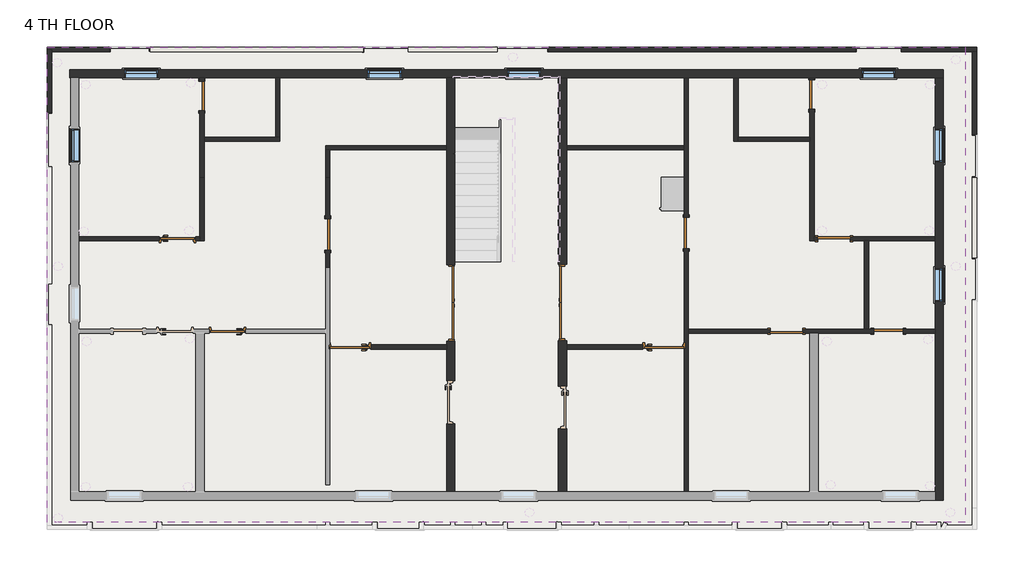
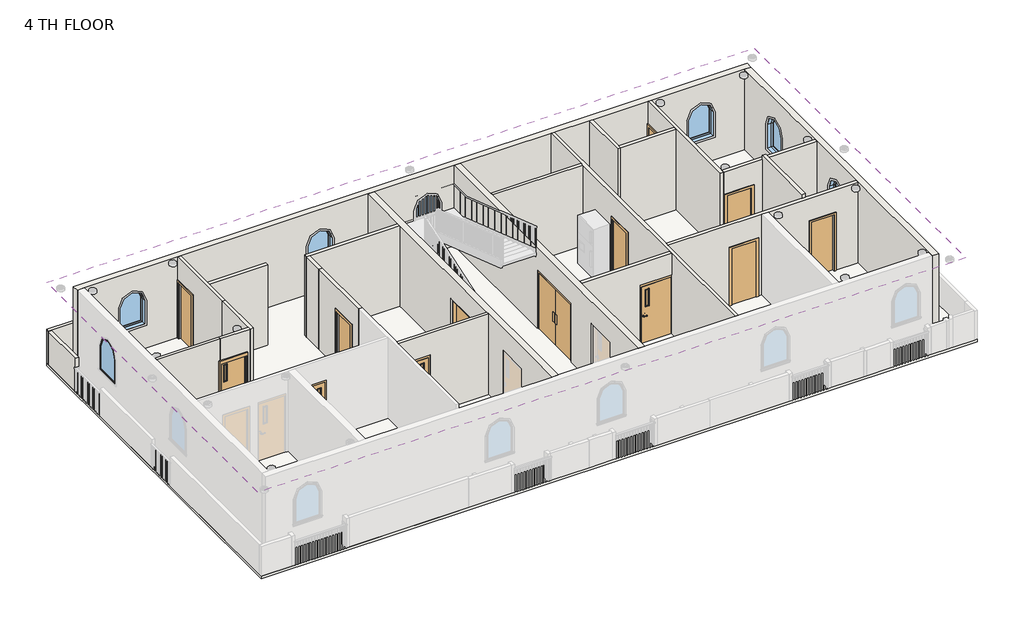
# One storey, part 2 of 7: 32 walls, 13 doors, 7 windows, 1 covering, 1 slab.
"""IFC4 building model written with IfcOpenShell, lengths in millimetres."""

from ifc_helpers import new_model, si_unit, frame, origin, place, context, project, spatial, polyline, circle_curve, outline, extrude, faceted_brep, transform, mapped, element, save
from ifc_brep_helpers import plane_surface, revolved_surface, advanced_brep
from components import door_2c854dd0, door_cf1f2706, door_4f5842df, door_passage_single_vision_lite_3_x7_440dd290, door_70e57c00, door_700d3439, door_8cb1b8a7, door_38851409, door_d141acb4, window_fixed_round_top_3_x_4_dee2be1c

model = new_model("IFC4")

# Units and contexts
model_context = context("Model", 3, world=origin())
ifc_project = project(units=[si_unit("LENGTHUNIT", "METRE", prefix="MILLI")], contexts=[model_context])

# Site, building, storey
site = spatial("IfcSite", under=ifc_project)
building = spatial("IfcBuilding", under=site)
storey = spatial("IfcBuildingStorey", under=building, Name="4 TH FLOOR", Elevation=12801.6)

# Covering
placement = place(None, origin())
element("IfcCovering", 1, ObjectType="2' x 4' ACT System", at=placement, inside=storey, context=model_context, shape_type="SweptSolid", body=[
    extrude(outline(polyline([(12235.5012075, 8470.0067329), (12235.5012075, -4623.6932193), (-13088.8067989, -4623.6932193), (-13088.8067989, 8470.0067329), (12235.5012075, 8470.0067329)])), frame((0.0, 0.0, 15849.6), z_axis=(0.0, 0.0, 1.0), x_axis=(1.0, 0.0, 0.0)), (0.0, 0.0, 1.0), 57.15),
])

# Doors
door_shape = door_2c854dd0(model_context)
element("IfcDoor", 2, ObjectType="Door-Passage-Double-Flush-Dbl_Acting : 6'79\" X 84\"", at=placement, inside=storey, context=model_context, shape_type="MappedRepresentation", body=[
    mapped(door_shape, transform((-1969.4487998, 1424.4578621, 12801.6), x_axis=(0.0, -1.0, 0.0), y_axis=(1.0, 0.0, 0.0), z_axis=(0.0, 0.0, 1.0))),
])
element("IfcDoor", 3, ObjectType="Door-Passage-Double-Flush-Dbl_Acting : 6'79\" X 84\"", at=placement, inside=storey, context=model_context, shape_type="MappedRepresentation", body=[
    mapped(door_shape, transform((1128.8432011, 1434.2067807, 12801.6), x_axis=(0.0, 1.0, 0.0), y_axis=(-1.0, 0.0, 0.0), z_axis=(0.0, 0.0, 1.0))),
])
door_2_shape = door_cf1f2706(model_context)
element("IfcDoor", 4, ObjectType="Door-Passage-Single-Vision_Lite : 3'6\"X7' 2", at=placement, inside=storey, context=model_context, shape_type="MappedRepresentation", body=[
    mapped(door_2_shape, transform((-4750.7487995, 211.6078621, 12801.6), x_axis=(-1.0, 0.0, 0.0), y_axis=(0.0, -1.0, 0.0), z_axis=(0.0, 0.0, 1.0))),
])
door_3_shape = door_4f5842df(model_context)
element("IfcDoor", 5, ObjectType="Door-Passage-Single-Vision_Lite : 3'6\"X7' 2", at=placement, inside=storey, context=model_context, shape_type="MappedRepresentation", body=[
    mapped(door_3_shape, transform((3923.3512082, 211.6078621, 12801.6), x_axis=(1.0, 0.0, 0.0), y_axis=(0.0, 1.0, 0.0), z_axis=(0.0, 0.0, 1.0))),
])
door_passage_single_vision_lite_3_x7_shape = door_passage_single_vision_lite_3_x7_440dd290(model_context)
element("IfcDoor", 6, ObjectType="Door-Passage-Single-Vision_Lite : 3'X7'", at=placement, inside=storey, context=model_context, shape_type="MappedRepresentation", body=[
    mapped(door_passage_single_vision_lite_3_x7_shape, transform((-9501.8462614, 3186.8067332, 12801.6), x_axis=(1.0, 0.0, 0.0), y_axis=(0.0, 1.0, 0.0), z_axis=(0.0, 0.0, 1.0))),
])
element("IfcDoor", 7, ObjectType="Door-Passage-Single-Vision_Lite : 3'X7'", at=placement, inside=storey, context=model_context, shape_type="MappedRepresentation", body=[
    mapped(door_passage_single_vision_lite_3_x7_shape, transform((-8122.5987992, 646.8067334, 12801.6), x_axis=(-1.0, 0.0, 0.0), y_axis=(0.0, -1.0, 0.0), z_axis=(0.0, 0.0, 1.0))),
])
door_4_shape = door_70e57c00(model_context)
element("IfcDoor", 8, ObjectType="Single-Flush : 2'10\" x 7'", at=placement, inside=storey, context=model_context, shape_type="MappedRepresentation", body=[
    mapped(door_4_shape, transform((-5360.3487995, 3313.8067802, 12801.6), x_axis=(0.0, -1.0, 0.0), y_axis=(1.0, 0.0, 0.0), z_axis=(0.0, 0.0, 1.0))),
])
door_5_shape = door_700d3439(model_context)
element("IfcDoor", 9, ObjectType="Single-Flush : 2'10\" x 7'", at=placement, inside=storey, context=model_context, shape_type="MappedRepresentation", body=[
    mapped(door_5_shape, transform((4532.9512082, 3351.906733, 12801.6), x_axis=(0.0, -1.0, 0.0), y_axis=(1.0, 0.0, 0.0), z_axis=(0.0, 0.0, 1.0))),
])
door_6_shape = door_8cb1b8a7(model_context)
element("IfcDoor", 10, ObjectType="Single-Flush : 2'11\"x 7'", at=placement, inside=storey, context=model_context, shape_type="MappedRepresentation", body=[
    mapped(door_6_shape, transform((8609.6512079, 3193.1567332, 12801.6), x_axis=(-1.0, 0.0, 0.0), y_axis=(0.0, -1.0, 0.0), z_axis=(0.0, 0.0, 1.0))),
])
element("IfcDoor", 11, ObjectType="Single-Flush : 2'11\"x 7'", at=placement, inside=storey, context=model_context, shape_type="MappedRepresentation", body=[
    mapped(door_6_shape, transform((7295.2012079, 640.4567334, 12801.6), x_axis=(1.0, 0.0, 0.0), y_axis=(0.0, 1.0, 0.0), z_axis=(0.0, 0.0, 1.0))),
])
door_7_shape = door_38851409(model_context)
element("IfcDoor", 12, ObjectType="Single-Flush : 2'8\"x 7'", at=placement, inside=storey, context=model_context, shape_type="MappedRepresentation", body=[
    mapped(door_7_shape, transform((-8827.4487992, 7136.5067329, 12801.6), x_axis=(0.0, 1.0, 0.0), y_axis=(-1.0, 0.0, 0.0), z_axis=(0.0, 0.0, 1.0))),
])
element("IfcDoor", 13, ObjectType="Single-Flush : 2'8\"x 7'", at=placement, inside=storey, context=model_context, shape_type="MappedRepresentation", body=[
    mapped(door_7_shape, transform((10111.5098918, 640.4567334, 12801.6), x_axis=(-1.0, 0.0, 0.0), y_axis=(0.0, -1.0, 0.0), z_axis=(0.0, 0.0, 1.0))),
])
door_8_shape = door_d141acb4(model_context)
element("IfcDoor", 14, ObjectType="Single-Flush : 2'8\"x 7'", at=placement, inside=storey, context=model_context, shape_type="MappedRepresentation", body=[
    mapped(door_8_shape, transform((8000.0512079, 7167.840939, 12801.6), x_axis=(0.0, 1.0, 0.0), y_axis=(-1.0, 0.0, 0.0), z_axis=(0.0, 0.0, 1.0))),
])

# Slab
element("IfcSlab", 15, ObjectType="LW Concrete on Metal Deck", at=placement, inside=storey, context=model_context, shape_type="SweptSolid", body=[
    extrude(outline(polyline([(12540.3012043, 8470.0067329), (12540.3012043, -4826.8932661), (-13088.8067989, -4826.8932661), (-13088.8067989, 8470.0067329), (12540.3012043, 8470.0067329)])), frame((0.0, 0.0, 12696.825), z_axis=(0.0, 0.0, 1.0), x_axis=(1.0, 0.0, 0.0)), (0.0, 0.0, 1.0), 104.775),
])

# Walls
element("IfcWall", 16, ObjectType="Generic - 4.5\"", at=placement, inside=storey, context=model_context, shape_type="SweptSolid", body=[
    extrude(outline(polyline([(15849.6, -9959.0462614), (15849.6, -12224.6987925), (12801.6, -12224.6987925), (12801.6, -10009.8462614), (15036.8, -10009.8462614), (15036.8, -9959.0462614), (15849.6, -9959.0462614)])), frame((0.0, 3136.0067332, 0.0), z_axis=(0.0, 1.0, 0.0), x_axis=(0.0, 0.0, 1.0)), (0.0, 0.0, 1.0), 114.3),
])
element("IfcWall", 17, ObjectType="Generic - 4.5\"", at=placement, inside=storey, context=model_context, shape_type="Brep", body=[
    faceted_brep([(-8884.5987992, 4875.906733, 12801.6), (-8884.5987992, 3250.3067332, 12801.6), (-8884.5987992, 3136.0067332, 12801.6), (-8884.5987992, 3136.0067332, 15849.6), (-8884.5987992, 3250.3067332, 15849.6), (-8884.5987992, 4875.906733, 15849.6), (-8770.2987992, 4875.906733, 12801.6), (-8770.2987992, 4875.906733, 15849.6), (-8770.2987992, 3136.0067332, 15849.6), (-8770.2987992, 3136.0067332, 12801.6)], [[[0, 1, 2, 3, 4, 5]], [[6, 7, 8, 9]], [[2, 1, 0, 6, 9]], [[5, 4, 3, 8, 7]], [[0, 5, 7, 6]], [[3, 2, 9, 8]]]),
])
element("IfcWall", 18, ObjectType="Generic - 4.5\"", at=placement, inside=storey, context=model_context, shape_type="SweptSolid", body=[
    extrude(outline(polyline([(15849.6, -2077.3987998), (15849.6, -5303.1987995), (15036.8, -5303.1987995), (15036.8, -4166.5487995), (12801.6, -4166.5487995), (12801.6, -2077.3987998), (15849.6, -2077.3987998)])), frame((0.0, 148.1078621, 0.0), z_axis=(0.0, 1.0, 0.0), x_axis=(0.0, 0.0, 1.0)), (0.0, 0.0, 1.0), 114.3),
])
element("IfcWall", 19, ObjectType="Generic - 4.5\"", at=placement, inside=storey, context=model_context, shape_type="Brep", body=[
    faceted_brep([(-2077.3987998, 5764.9067329, 12801.6), (-5417.4987995, 5764.9067329, 12801.6), (-5417.4987995, 5764.9067329, 15849.6), (-2077.3987998, 5764.9067329, 15849.6), (-2077.3987998, 5650.6067329, 12801.6), (-2077.3987998, 5650.6067329, 15849.6), (-5303.1987995, 5650.6067329, 15849.6), (-5417.4987995, 5650.6067329, 15849.6), (-5417.4987995, 5650.6067329, 12801.6), (-5303.1987995, 5650.6067329, 12801.6)], [[[0, 1, 2, 3]], [[4, 5, 6, 7, 8, 9]], [[1, 0, 4, 9, 8]], [[3, 2, 7, 6, 5]], [[2, 1, 8, 7]], [[0, 3, 5, 4]]]),
])
element("IfcWall", 20, ObjectType="Generic - 4.5\"", at=placement, inside=storey, context=model_context, shape_type="SweptSolid", body=[
    extrude(outline(polyline([(-5417.4987995, 4875.90678), (-5417.4987995, 5650.6067329), (-5303.1987995, 5650.6067329), (-5303.1987995, 4875.90678), (-5417.4987995, 4875.90678)])), frame((0.0, 0.0, 12801.6), z_axis=(0.0, 0.0, 1.0), x_axis=(1.0, 0.0, 0.0)), (0.0, 0.0, 1.0), 3048.0),
])
element("IfcWall", 21, ObjectType="Generic - 4.5\"", at=placement, inside=storey, context=model_context, shape_type="SweptSolid", body=[
    extrude(outline(polyline([(4475.8012082, 5650.6067329), (1250.0012085, 5650.6067329), (1250.0012085, 5764.9067329), (4475.8012082, 5764.9067329), (4475.8012082, 5650.6067329)])), frame((0.0, 0.0, 12801.6), z_axis=(0.0, 0.0, 1.0), x_axis=(1.0, 0.0, 0.0)), (0.0, 0.0, 1.0), 3048.0),
])
element("IfcWall", 22, ObjectType="Generic - 4.5\"", at=placement, inside=storey, context=model_context, shape_type="Brep", body=[
    faceted_brep([(4475.8012082, -3785.4932193, 15849.6), (4475.8012082, 148.1078621, 15849.6), (4475.8012082, 262.4078621, 15849.6), (4475.8012082, 5650.6067329, 15849.6), (4475.8012082, 5764.9067329, 15849.6), (4475.8012082, 7631.8067329, 15849.6), (4475.8012082, 7631.8067329, 12801.6), (4475.8012082, 5764.9067329, 12801.6), (4475.8012082, 5650.6067329, 12801.6), (4475.8012082, 3783.706733, 12801.6), (4475.8012082, 3783.706733, 14935.2), (4475.8012082, 2920.106733, 14935.2), (4475.8012082, 2920.106733, 12801.6), (4475.8012082, 262.4078621, 12801.6), (4475.8012082, 262.4078621, 15036.8), (4475.8012082, 148.1078621, 15036.8), (4475.8012082, 148.1078621, 12801.6), (4475.8012082, -3785.4932193, 12801.6), (4590.1012082, 7631.8067329, 15849.6), (4590.1012082, 697.6067334, 15849.6), (4590.1012082, 583.3067334, 15849.6), (4590.1012082, -3785.4932193, 15849.6), (4590.1012082, -3785.4932193, 12801.6), (4590.1012082, 583.3067334, 12801.6), (4590.1012082, 697.6067334, 12801.6), (4590.1012082, 2920.106733, 12801.6), (4590.1012082, 2920.106733, 14935.2), (4590.1012082, 3783.706733, 14935.2), (4590.1012082, 3783.706733, 12801.6), (4590.1012082, 7631.8067329, 12801.6), (4507.5512082, 148.1078621, 12801.6), (4507.5512082, 262.4078621, 12801.6), (4507.5512082, 148.1078621, 15036.8), (4507.5512082, 262.4078621, 15036.8)], [[[0, 1, 2, 3, 4, 5, 6, 7, 8, 9, 10, 11, 12, 13, 14, 15, 16, 17]], [[18, 19, 20, 21, 22, 23, 24, 25, 26, 27, 28, 29]], [[6, 29, 28, 9, 8, 7]], [[12, 25, 24, 23, 22, 17, 16, 30, 31, 13]], [[5, 4, 3, 2, 1, 0, 21, 20, 19, 18]], [[6, 5, 18, 29]], [[28, 27, 10, 9]], [[27, 26, 11, 10]], [[26, 25, 12, 11]], [[0, 17, 22, 21]], [[32, 30, 16, 15]], [[31, 33, 14, 13]], [[30, 32, 33, 31]], [[33, 32, 15, 14]]]),
])
element("IfcWall", 23, ObjectType="Generic - 4.5\"", at=placement, inside=storey, context=model_context, shape_type="Brep", body=[
    faceted_brep([(5847.401208, 7631.8067329, 12801.6), (5847.401208, 5879.2067329, 12801.6), (5847.401208, 5879.2067329, 15849.6), (5847.401208, 7631.8067329, 15849.6), (5961.701208, 7631.8067329, 12801.6), (5961.701208, 7631.8067329, 15849.6), (5961.701208, 5993.5067329, 15849.6), (5961.701208, 5879.2067329, 15849.6), (5961.701208, 5879.2067329, 12801.6), (5961.701208, 5993.5067329, 12801.6)], [[[0, 1, 2, 3]], [[4, 5, 6, 7, 8, 9]], [[1, 0, 4, 9, 8]], [[3, 2, 7, 6, 5]], [[0, 3, 5, 4]], [[2, 1, 8, 7]]]),
])
element("IfcWall", 24, ObjectType="Generic - 4.5\"", at=placement, inside=storey, context=model_context, shape_type="SweptSolid", body=[
    extrude(outline(polyline([(7942.9012079, 5879.2067329), (5961.701208, 5879.2067329), (5961.701208, 5993.5067329), (7942.9012079, 5993.5067329), (7942.9012079, 5879.2067329)])), frame((0.0, 0.0, 12801.6), z_axis=(0.0, 0.0, 1.0), x_axis=(1.0, 0.0, 0.0)), (0.0, 0.0, 1.0), 3048.0),
])
element("IfcWall", 25, ObjectType="Generic - 4.5\"", at=placement, inside=storey, context=model_context, shape_type="Brep", body=[
    faceted_brep([(7942.9012079, 7625.040939, 12801.6), (7942.9012079, 7574.240939, 12801.6), (7942.9012079, 7574.240939, 14935.2), (7942.9012079, 6761.440939, 14935.2), (7942.9012079, 6761.440939, 12801.6), (7942.9012079, 5993.5067329, 12801.6), (7942.9012079, 5879.2067329, 12801.6), (7942.9012079, 3136.0067332, 12801.6), (7942.9012079, 3136.0067332, 15849.6), (7942.9012079, 5879.2067329, 15849.6), (7942.9012079, 5993.5067329, 15849.6), (7942.9012079, 7625.040939, 15849.6), (8057.2012079, 7574.240939, 14935.2), (8057.2012079, 7574.240939, 12801.6), (8057.2012079, 7625.040939, 12801.6), (8057.2012079, 7625.040939, 15849.6), (8057.2012079, 3250.3067332, 15849.6), (8057.2012079, 3136.0067332, 15849.6), (8057.2012079, 3136.0067332, 12801.6), (8057.2012079, 3250.3067332, 12801.6), (8057.2012079, 6761.440939, 12801.6), (8057.2012079, 6761.440939, 14935.2)], [[[0, 1, 2, 3, 4, 5, 6, 7, 8, 9, 10, 11]], [[12, 13, 14, 15, 16, 17, 18, 19, 20, 21]], [[14, 13, 1, 0]], [[20, 19, 18, 7, 6, 5, 4]], [[11, 10, 9, 8, 17, 16, 15]], [[0, 11, 15, 14]], [[8, 7, 18, 17]], [[2, 1, 13, 12]], [[3, 2, 12, 21]], [[4, 3, 21, 20]]]),
])
element("IfcWall", 26, ObjectType="Generic - 4.5\"", at=placement, inside=storey, context=model_context, shape_type="Brep", body=[
    faceted_brep([(8165.1512079, 3250.3067332, 14935.2), (8165.1512079, 3250.3067332, 12801.6), (8057.2012079, 3250.3067332, 12801.6), (8057.2012079, 3250.3067332, 15849.6), (11397.3012075, 3250.3067332, 15849.6), (11397.3012075, 3250.3067332, 12801.6), (9054.1512079, 3250.3067332, 12801.6), (9054.1512079, 3250.3067332, 14935.2), (8057.2012079, 3136.0067332, 12801.6), (8165.1512079, 3136.0067332, 12801.6), (8165.1512079, 3136.0067332, 14935.2), (9054.1512079, 3136.0067332, 14935.2), (9054.1512079, 3136.0067332, 12801.6), (9438.4098918, 3136.0067332, 12801.6), (9565.4098918, 3136.0067332, 12801.6), (11397.3012075, 3136.0067332, 12801.6), (11397.3012075, 3136.0067332, 15849.6), (8057.2012079, 3136.0067332, 15849.6)], [[[0, 1, 2, 3, 4, 5, 6, 7]], [[8, 9, 10, 11, 12, 13, 14, 15, 16, 17]], [[6, 5, 15, 14, 13, 12]], [[2, 1, 9, 8]], [[4, 3, 17, 16]], [[3, 2, 8, 17]], [[5, 4, 16, 15]], [[10, 9, 1, 0]], [[11, 10, 0, 7]], [[12, 11, 7, 6]]]),
])
element("IfcWall", 27, ObjectType="Generic - 4.5\"", at=placement, inside=storey, context=model_context, shape_type="Brep", body=[
    faceted_brep([(7739.7012079, 583.3067334, 14935.2), (7739.7012079, 583.3067334, 12801.6), (7942.9012079, 583.3067334, 12801.6), (8171.5012079, 583.3067334, 12801.6), (9705.1098918, 583.3067334, 12801.6), (9705.1098918, 583.3067334, 14935.2), (10517.9098918, 583.3067334, 14935.2), (10517.9098918, 583.3067334, 12801.6), (11397.3012075, 583.3067334, 12801.6), (11397.3012075, 583.3067334, 15849.6), (8171.5012079, 583.3067334, 15849.6), (7942.9012079, 583.3067334, 15849.6), (4590.1012082, 583.3067334, 15849.6), (4590.1012082, 583.3067334, 12801.6), (6850.7012079, 583.3067334, 12801.6), (6850.7012079, 583.3067334, 14935.2), (9705.1098918, 697.6067334, 12801.6), (9565.4098918, 697.6067334, 12801.6), (9438.4098918, 697.6067334, 12801.6), (7739.7012079, 697.6067334, 12801.6), (7739.7012079, 697.6067334, 14935.2), (6850.7012079, 697.6067334, 14935.2), (6850.7012079, 697.6067334, 12801.6), (4590.1012082, 697.6067334, 12801.6), (4590.1012082, 697.6067334, 15849.6), (11397.3012075, 697.6067334, 15849.6), (11397.3012075, 697.6067334, 12801.6), (10517.9098918, 697.6067334, 12801.6), (10517.9098918, 697.6067334, 14935.2), (9705.1098918, 697.6067334, 14935.2)], [[[0, 1, 2, 3, 4, 5, 6, 7, 8, 9, 10, 11, 12, 13, 14, 15]], [[16, 17, 18, 19, 20, 21, 22, 23, 24, 25, 26, 27, 28, 29]], [[27, 26, 8, 7]], [[14, 13, 23, 22]], [[4, 3, 2, 1, 19, 18, 17, 16]], [[12, 11, 10, 9, 25, 24]], [[9, 8, 26, 25]], [[13, 12, 24, 23]], [[5, 4, 16, 29]], [[6, 5, 29, 28]], [[7, 6, 28, 27]], [[20, 19, 1, 0]], [[21, 20, 0, 15]], [[22, 21, 15, 14]]]),
])
element("IfcWall", 28, ObjectType="Generic - 4.5\"", at=placement, inside=storey, context=model_context, shape_type="Brep", body=[
    faceted_brep([(-8770.2987992, 7542.9067329, 14935.2), (-8770.2987992, 7542.9067329, 12801.6), (-8770.2987992, 7631.8067329, 12801.6), (-8770.2987992, 7631.8067329, 15849.6), (-8770.2987992, 5993.5067329, 15849.6), (-8770.2987992, 5879.2067329, 15849.6), (-8770.2987992, 4875.906733, 15849.6), (-8770.2987992, 4875.906733, 12801.6), (-8770.2987992, 5879.2067329, 12801.6), (-8770.2987992, 5993.5067329, 12801.6), (-8770.2987992, 6730.1067329, 12801.6), (-8770.2987992, 6730.1067329, 14935.2), (-8884.5987992, 7631.8067329, 12801.6), (-8884.5987992, 7542.9067329, 12801.6), (-8884.5987992, 7542.9067329, 14935.2), (-8884.5987992, 6730.1067329, 14935.2), (-8884.5987992, 6730.1067329, 12801.6), (-8884.5987992, 4875.906733, 12801.6), (-8884.5987992, 4875.906733, 15849.6), (-8884.5987992, 7631.8067329, 15849.6)], [[[0, 1, 2, 3, 4, 5, 6, 7, 8, 9, 10, 11]], [[12, 13, 14, 15, 16, 17, 18, 19]], [[2, 1, 13, 12]], [[10, 9, 8, 7, 17, 16]], [[6, 5, 4, 3, 19, 18]], [[7, 6, 18, 17]], [[3, 2, 12, 19]], [[14, 13, 1, 0]], [[15, 14, 0, 11]], [[16, 15, 11, 10]]]),
])
element("IfcWall", 29, ObjectType="Generic - 4.5\"", at=placement, inside=storey, context=model_context, shape_type="Brep", body=[
    faceted_brep([(-8770.2987992, 5879.2067329, 12801.6), (-6674.7987994, 5879.2067329, 12801.6), (-6674.7987994, 5879.2067329, 15849.6), (-8770.2987992, 5879.2067329, 15849.6), (-8770.2987992, 5993.5067329, 12801.6), (-8770.2987992, 5993.5067329, 15849.6), (-6674.7987994, 5993.5067329, 15849.6), (-6674.7987994, 5993.5067329, 14173.2), (-6674.7987994, 5993.5067329, 12801.6), (-6789.0987994, 5993.5067329, 12801.6)], [[[0, 1, 2, 3]], [[4, 5, 6, 7, 8, 9]], [[1, 0, 4, 9, 8]], [[3, 2, 6, 5]], [[0, 3, 5, 4]], [[2, 1, 8, 7, 6]]]),
])
element("IfcWall", 30, ObjectType="Generic - 4.5\"", at=placement, inside=storey, context=model_context, shape_type="SweptSolid", body=[
    extrude(outline(polyline([(-6674.7987994, 7631.8067329), (-6674.7987994, 5993.5067329), (-6789.0987994, 5993.5067329), (-6789.0987994, 7631.8067329), (-6674.7987994, 7631.8067329)])), frame((0.0, 0.0, 12801.6), z_axis=(0.0, 0.0, 1.0), x_axis=(1.0, 0.0, 0.0)), (0.0, 0.0, 1.0), 1371.6),
])
element("IfcWall", 31, ObjectType="Generic - 4.5\"", at=placement, inside=storey, context=model_context, shape_type="SweptSolid", body=[
    extrude(outline(polyline([(15849.6, -8884.5987992), (15849.6, -9959.0462614), (15036.8, -9959.0462614), (15036.8, -8993.8462614), (12801.6, -8993.8462614), (12801.6, -8884.5987992), (15849.6, -8884.5987992)])), frame((0.0, 3136.0067332, 0.0), z_axis=(0.0, 1.0, 0.0), x_axis=(0.0, 0.0, 1.0)), (0.0, 0.0, 1.0), 114.3),
])
element("IfcWall", 32, ObjectType="Generic - 4.5\"", at=placement, inside=storey, context=model_context, shape_type="SweptSolid", body=[
    extrude(outline(polyline([(2882.0067802, 14935.2), (2882.0067802, 12801.6), (2399.4067802, 12801.6), (2399.4067802, 15849.6), (4875.90678, 15849.6), (4875.90678, 12801.6), (3745.6067802, 12801.6), (3745.6067802, 14935.2), (2882.0067802, 14935.2)])), frame((-5417.4987995, 0.0, 0.0), z_axis=(1.0, 0.0, 0.0), x_axis=(0.0, 1.0, 0.0)), (0.0, 0.0, 1.0), 114.3),
])
element("IfcWall", 33, ObjectType="Generic - 4.5\"", at=placement, inside=storey, context=model_context, shape_type="SweptSolid", body=[
    extrude(outline(polyline([(15849.6, 4475.8012082), (15849.6, 1250.0012085), (12801.6, 1250.0012085), (12801.6, 3339.1512082), (15036.8, 3339.1512082), (15036.8, 4475.8012082), (15849.6, 4475.8012082)])), frame((0.0, 148.1078621, 0.0), z_axis=(0.0, 1.0, 0.0), x_axis=(0.0, 0.0, 1.0)), (0.0, 0.0, 1.0), 114.3),
])
element("IfcWall", 34, ObjectType="Generic - 4.5\"", at=placement, inside=storey, context=model_context, shape_type="SweptSolid", body=[
    extrude(outline(polyline([(-12973.9987925, 8412.8567329), (-12973.9987925, 6682.2711337), (-13088.2987925, 6682.2711337), (-13088.2987925, 8412.8567329), (-12973.9987925, 8412.8567329)])), frame((0.0, 0.0, 12801.6), z_axis=(0.0, 0.0, 1.0), x_axis=(1.0, 0.0, 0.0)), (0.0, 0.0, 1.0), 1259.0059812),
])
element("IfcWall", 35, ObjectType="Generic - 4.5\"", at=placement, inside=storey, context=model_context, shape_type="SweptSolid", body=[
    extrude(outline(polyline([(-11387.0067989, 8355.7067329), (-13088.8067989, 8355.7067329), (-13088.8067989, 8470.0067329), (-11387.0067989, 8470.0067329), (-11387.0067989, 8355.7067329)])), frame((0.0, 0.0, 12801.6), z_axis=(0.0, 0.0, 1.0), x_axis=(1.0, 0.0, 0.0)), (0.0, 0.0, 1.0), 1273.4134002),
])
element("IfcWall", 36, ObjectType="Generic - 4.5\"", at=placement, inside=storey, context=model_context, shape_type="SweptSolid", body=[
    extrude(outline(polyline([(-4382.4487992, 8355.7067329), (-10247.1817989, 8355.7067329), (-10247.1817989, 8470.0067329), (-4382.4487992, 8470.0067329), (-4382.4487992, 8355.7067329)])), frame((0.0, 0.0, 12801.6), z_axis=(0.0, 0.0, 1.0), x_axis=(1.0, 0.0, 0.0)), (0.0, 0.0, 1.0), 1083.89837),
])
element("IfcWall", 37, ObjectType="Generic - 4.5\"", at=placement, inside=storey, context=model_context, shape_type="SweptSolid", body=[
    extrude(outline(polyline([(-682.0490672, 8355.7067329), (-3139.4990672, 8355.7067329), (-3139.4990672, 8470.0067329), (-682.0490672, 8470.0067329), (-682.0490672, 8355.7067329)])), frame((0.0, 0.0, 12801.6), z_axis=(0.0, 0.0, 1.0), x_axis=(1.0, 0.0, 0.0)), (0.0, 0.0, 1.0), 1195.9732529),
])
element("IfcWall", 38, ObjectType="Generic - 4.5\"", at=placement, inside=storey, context=model_context, shape_type="SweptSolid", body=[
    extrude(outline(polyline([(9199.6932011, 8355.7067329), (741.4932011, 8355.7067329), (741.4932011, 8470.0067329), (9199.6932011, 8470.0067329), (9199.6932011, 8355.7067329)])), frame((0.0, 0.0, 12801.6), z_axis=(0.0, 0.0, 1.0), x_axis=(1.0, 0.0, 0.0)), (0.0, 0.0, 1.0), 1274.1868366),
])
element("IfcWall", 39, ObjectType="Generic - 4.5\"", at=placement, inside=storey, context=model_context, shape_type="Brep", body=[
    faceted_brep([(10462.2009401, 8355.7067329, 12801.6), (12426.0012043, 8355.7067329, 12801.6), (12540.3012043, 8355.7067329, 12801.6), (12540.3012043, 8355.7067329, 14167.3502881), (10462.2009401, 8355.7067329, 14167.3502881), (10462.2009401, 8470.0067329, 12801.6), (10462.2009401, 8470.0067329, 14167.3502881), (12540.3012043, 8470.0067329, 14167.3502881), (12540.3012043, 8470.0067329, 12801.6)], [[[0, 1, 2, 3, 4]], [[5, 6, 7, 8]], [[2, 1, 0, 5, 8]], [[4, 3, 7, 6]], [[0, 4, 6, 5]], [[3, 2, 8, 7]]]),
])
element("IfcWall", 40, ObjectType="Generic - 4.5\"", at=placement, inside=storey, context=model_context, shape_type="Brep", body=[
    faceted_brep([(12426.0012043, 8355.7067329, 12801.6), (12426.0012043, 6069.7067329, 12801.6), (12426.0012043, 6069.7067329, 14173.2), (12426.0012043, 8355.7067329, 14173.2), (12540.3012043, 8355.7067329, 12801.6), (12540.3012043, 8355.7067329, 14167.3502881), (12540.3012043, 8355.7067329, 14173.2), (12540.3012043, 6069.7067329, 14173.2), (12540.3012043, 6069.7067329, 12801.6)], [[[0, 1, 2, 3]], [[4, 5, 6, 7, 8]], [[1, 0, 4, 8]], [[2, 1, 8, 7]], [[3, 2, 7, 6]], [[0, 3, 6, 5, 4]]]),
])
element("IfcWall", 41, ObjectType="Generic - 4.5\"", at=placement, inside=storey, context=model_context, shape_type="SweptSolid", body=[
    extrude(outline(polyline([(12426.0012043, 2666.1067329), (12426.0012043, 4875.9067329), (12540.3012043, 4875.9067329), (12540.3012043, 2666.1067329), (12426.0012043, 2666.1067329)])), frame((0.0, 0.0, 12801.6), z_axis=(0.0, 0.0, 1.0), x_axis=(1.0, 0.0, 0.0)), (0.0, 0.0, 1.0), 1193.0409005),
])
element("IfcWall", 42, ObjectType="Generic - 9\"", at=placement, inside=storey, context=model_context, shape_type="AdvancedBrep", body=[
    advanced_brep(
    [(-12479.2067989, 7631.8067329, 12801.6), (-12453.2987925, 7631.8067329, 12801.6), (-12224.6987925, 7631.8067329, 12801.6), (-8884.5987992, 7631.8067329, 12801.6), (-8770.2987992, 7631.8067329, 12801.6), (-6789.0987994, 7631.8067329, 12801.6), (-6674.7987994, 7631.8067329, 12801.6), (-2077.3987998, 7631.8067329, 12801.6), (-1848.7987998, 7631.8067329, 12801.6), (1008.1932011, 7631.8067329, 12801.6), (1236.7932011, 7631.8067329, 12801.6), (4475.8012082, 7631.8067329, 12801.6), (4590.1012082, 7631.8067329, 12801.6), (5847.401208, 7631.8067329, 12801.6), (5961.701208, 7631.8067329, 12801.6), (11397.3012075, 7631.8067329, 12801.6), (11625.9012075, 7631.8067329, 12801.6), (11625.9012075, 7631.8067329, 15849.6), (11397.3012075, 7631.8067329, 15849.6), (5961.701208, 7631.8067329, 15849.6), (5847.401208, 7631.8067329, 15849.6), (4590.1012082, 7631.8067329, 15849.6), (4475.8012082, 7631.8067329, 15849.6), (1236.7932011, 7631.8067329, 15849.6), (1008.1932011, 7631.8067329, 15849.6), (-1848.7987998, 7631.8067329, 15849.6), (-2077.3987998, 7631.8067329, 15849.6), (-8770.2987992, 7631.8067329, 15849.6), (-8884.5987992, 7631.8067329, 15849.6), (-12224.6987925, 7631.8067329, 15849.6), (-12453.2987925, 7631.8067329, 15849.6), (-12479.2067989, 7631.8067329, 15849.6), (9378.0012075, 7631.8067329, 13716.0), (9378.0012075, 7631.8067329, 14630.4), (10292.4012075, 7631.8067329, 14630.4), (10292.4012075, 7631.8067329, 13716.0), (-401.5067989, 7631.8067329, 13716.0), (-401.5067989, 7631.8067329, 14630.4), (512.8932011, 7631.8067329, 14630.4), (512.8932011, 7631.8067329, 13716.0), (-4249.0987998, 7631.8067329, 13716.0), (-4249.0987998, 7631.8067329, 14630.4), (-3334.6987998, 7631.8067329, 14630.4), (-3334.6987998, 7631.8067329, 13716.0), (-10961.0487992, 7631.8067329, 13716.0), (-10961.0487992, 7631.8067329, 14630.4), (-10046.6487992, 7631.8067329, 14630.4), (-10046.6487992, 7631.8067329, 13716.0), (-12479.2067989, 7860.4067329, 12801.6), (-12479.2067989, 7860.4067329, 15849.6), (11625.9012075, 7860.4067329, 15849.6), (11625.9012075, 7860.4067329, 12801.6), (9378.0012075, 7860.4067329, 13716.0), (10292.4012075, 7860.4067329, 13716.0), (10292.4012075, 7860.4067329, 14630.4), (9378.0012075, 7860.4067329, 14630.4), (-401.5067989, 7860.4067329, 13716.0), (512.8932011, 7860.4067329, 13716.0), (512.8932011, 7860.4067329, 14630.4), (-401.5067989, 7860.4067329, 14630.4), (-4249.0987998, 7860.4067329, 13716.0), (-3334.6987998, 7860.4067329, 13716.0), (-3334.6987998, 7860.4067329, 14630.4), (-4249.0987998, 7860.4067329, 14630.4), (-10961.0487992, 7860.4067329, 13716.0), (-10046.6487992, 7860.4067329, 13716.0), (-10046.6487992, 7860.4067329, 14630.4), (-10961.0487992, 7860.4067329, 14630.4)],
    [
        (0, 1),
        (1, 2),
        (2, 3),
        (3, 4),
        (4, 5),
        (5, 6),
        (6, 7),
        (7, 8),
        (8, 9),
        (9, 10),
        (10, 11),
        (11, 12),
        (12, 13),
        (13, 14),
        (14, 15),
        (15, 16),
        (16, 17),
        (17, 18),
        (18, 19),
        (19, 20),
        (20, 21),
        (21, 22),
        (22, 23),
        (23, 24),
        (24, 25),
        (25, 26),
        (26, 27),
        (27, 28),
        (28, 29),
        (29, 30),
        (30, 31),
        (31, 0),
        (32, 33),
        (33, 34, circle_curve(frame((9835.2012075, 7631.8067329, 14630.4), z_axis=(0.0, 1.0, 0.0), x_axis=(1.0, 0.0, 0.0)), 457.2)),
        (34, 35),
        (35, 32),
        (36, 37),
        (37, 38, circle_curve(frame((55.6932011, 7631.8067329, 14630.4), z_axis=(0.0, 1.0, 0.0), x_axis=(1.0, 0.0, 0.0)), 457.2)),
        (38, 39),
        (39, 36),
        (40, 41),
        (41, 42, circle_curve(frame((-3791.8987998, 7631.8067329, 14630.4), z_axis=(0.0, 1.0, 0.0), x_axis=(1.0, 0.0, 0.0)), 457.2)),
        (42, 43),
        (43, 40),
        (44, 45),
        (45, 46, circle_curve(frame((-10503.8487992, 7631.8067329, 14630.4), z_axis=(0.0, 1.0, 0.0), x_axis=(1.0, 0.0, 0.0)), 457.2)),
        (46, 47),
        (47, 44),
        (48, 49),
        (49, 50),
        (50, 51),
        (51, 48),
        (52, 53),
        (53, 54),
        (54, 55, circle_curve(frame((9835.2012075, 7860.4067329, 14630.4), z_axis=(0.0, -1.0, 0.0), x_axis=(1.0, 0.0, 0.0)), 457.2)),
        (55, 52),
        (56, 57),
        (57, 58),
        (58, 59, circle_curve(frame((55.6932011, 7860.4067329, 14630.4), z_axis=(0.0, -1.0, 0.0), x_axis=(1.0, 0.0, 0.0)), 457.2)),
        (59, 56),
        (60, 61),
        (61, 62),
        (62, 63, circle_curve(frame((-3791.8987998, 7860.4067329, 14630.4), z_axis=(0.0, -1.0, 0.0), x_axis=(1.0, 0.0, 0.0)), 457.2)),
        (63, 60),
        (64, 65),
        (65, 66),
        (66, 67, circle_curve(frame((-10503.8487992, 7860.4067329, 14630.4), z_axis=(0.0, -1.0, 0.0), x_axis=(1.0, 0.0, 0.0)), 457.2)),
        (67, 64),
        (0, 48),
        (51, 16),
        (17, 50),
        (49, 31),
        (52, 32),
        (35, 53),
        (34, 54),
        (33, 55),
        (56, 36),
        (39, 57),
        (38, 58),
        (37, 59),
        (60, 40),
        (43, 61),
        (42, 62),
        (41, 63),
        (64, 44),
        (47, 65),
        (46, 66),
        (45, 67),
    ],
    [
        plane_surface(frame((-12479.2067989, 7631.8067329, 12801.6), z_axis=(0.0, -1.0, 0.0), x_axis=(1.0, 0.0, 0.0))),
        plane_surface(frame((-12479.2067989, 7860.4067329, 12801.6), z_axis=(0.0, 1.0, 0.0), x_axis=(-1.0, 0.0, 0.0))),
        plane_surface(frame((-12479.2067989, 7631.8067329, 12801.6), z_axis=(0.0, 0.0, -1.0), x_axis=(0.0, 1.0, 0.0))),
        plane_surface(frame((11511.6012075, 7631.8067329, 15849.6), z_axis=(0.0, 0.0, 1.0), x_axis=(0.0, 1.0, 0.0))),
        plane_surface(frame((-12479.2067989, 7631.8067329, 15849.6), z_axis=(-1.0, 0.0, 0.0), x_axis=(0.0, 1.0, 0.0))),
        plane_surface(frame((11625.9012075, 7629.6366753, 12801.6), z_axis=(1.0, 0.0, 0.0), x_axis=(0.0, 1.0, 0.0))),
        plane_surface(frame((9378.0012075, 7860.4067329, 13716.0), z_axis=(0.0, 0.0, 1.0), x_axis=(0.0, -1.0, 0.0))),
        plane_surface(frame((10292.4012075, 7860.4067329, 13716.0), z_axis=(-1.0, 0.0, 0.0), x_axis=(0.0, -1.0, 0.0))),
        revolved_surface(polyline([(10292.401207500001, 7631.8067329, 14630.4), (10292.401207500001, 7860.4067329, 14630.4)]), (9835.2012075, 7631.8067329, 14630.4), (0.0, -1.0, 0.0)),
        plane_surface(frame((9378.0012075, 7860.4067329, 14630.4), z_axis=(1.0, 0.0, 0.0), x_axis=(0.0, -1.0, 0.0))),
        plane_surface(frame((-401.5067989, 7860.4067329, 13716.0), z_axis=(0.0, 0.0, 1.0), x_axis=(0.0, -1.0, 0.0))),
        plane_surface(frame((512.8932011, 7860.4067329, 13716.0), z_axis=(-1.0, 0.0, 0.0), x_axis=(0.0, -1.0, 0.0))),
        revolved_surface(polyline([(512.8932010999999, 7631.8067329, 14630.4), (512.8932010999999, 7860.4067329, 14630.4)]), (55.6932011, 7631.8067329, 14630.4), (0.0, -1.0, 0.0)),
        plane_surface(frame((-401.5067989, 7860.4067329, 14630.4), z_axis=(1.0, 0.0, 0.0), x_axis=(0.0, -1.0, 0.0))),
        plane_surface(frame((-4249.0987998, 7860.4067329, 13716.0), z_axis=(0.0, 0.0, 1.0), x_axis=(0.0, -1.0, 0.0))),
        plane_surface(frame((-3334.6987998, 7860.4067329, 13716.0), z_axis=(-1.0, 0.0, 0.0), x_axis=(0.0, -1.0, 0.0))),
        revolved_surface(polyline([(-3334.6987998, 7631.8067329, 14630.4), (-3334.6987998, 7860.4067329, 14630.4)]), (-3791.8987998, 7631.8067329, 14630.4), (0.0, -1.0, 0.0)),
        plane_surface(frame((-4249.0987998, 7860.4067329, 14630.4), z_axis=(1.0, 0.0, 0.0), x_axis=(0.0, -1.0, 0.0))),
        plane_surface(frame((-10961.0487992, 7860.4067329, 13716.0), z_axis=(0.0, 0.0, 1.0), x_axis=(0.0, -1.0, 0.0))),
        plane_surface(frame((-10046.6487992, 7860.4067329, 13716.0), z_axis=(-1.0, 0.0, 0.0), x_axis=(0.0, -1.0, 0.0))),
        revolved_surface(polyline([(-10046.648799199998, 7631.8067329, 14630.4), (-10046.648799199998, 7860.4067329, 14630.4)]), (-10503.8487992, 7631.8067329, 14630.4), (0.0, -1.0, 0.0)),
        plane_surface(frame((-10961.0487992, 7860.4067329, 14630.4), z_axis=(1.0, 0.0, 0.0), x_axis=(0.0, -1.0, 0.0))),
    ],
    [
        (0, [[1, 2, 3, 4, 5, 6, 7, 8, 9, 10, 11, 12, 13, 14, 15, 16, 17, 18, 19, 20, 21, 22, 23, 24, 25, 26, 27, 28, 29, 30, 31, 32], [33, 34, 35, 36], [37, 38, 39, 40], [41, 42, 43, 44], [45, 46, 47, 48]]),
        (1, [[49, 50, 51, 52], [53, 54, 55, 56], [57, 58, 59, 60], [61, 62, 63, 64], [65, 66, 67, 68]]),
        (2, [[-16, -15, -14, -13, -12, -11, -10, -9, -8, -7, -6, -5, -4, -3, -2, -1, 69, -52, 70]]),
        (3, [[-31, -30, -29, -28, -27, -26, -25, -24, -23, -22, -21, -20, -19, -18, 71, -50, 72]]),
        (4, [[-32, -72, -49, -69]]),
        (5, [[-17, -70, -51, -71]]),
        (6, [[-53, 73, -36, 74]]),
        (7, [[-54, -74, -35, 75]]),
        (8, [[-55, -75, -34, 76]]),
        (9, [[-56, -76, -33, -73]]),
        (10, [[-57, 77, -40, 78]]),
        (11, [[-58, -78, -39, 79]]),
        (12, [[-59, -79, -38, 80]]),
        (13, [[-60, -80, -37, -77]]),
        (14, [[-61, 81, -44, 82]]),
        (15, [[-62, -82, -43, 83]]),
        (16, [[-63, -83, -42, 84]]),
        (17, [[-64, -84, -41, -81]]),
        (18, [[-65, 85, -48, 86]]),
        (19, [[-66, -86, -47, 87]]),
        (20, [[-67, -87, -46, 88]]),
        (21, [[-68, -88, -45, -85]]),
    ],
),
])
element("IfcWall", 43, ObjectType="Generic - 9\"", at=placement, inside=storey, context=model_context, shape_type="AdvancedBrep", body=[
    advanced_brep(
    [(11397.3012075, 7631.8067329, 12801.6), (11397.3012075, 3250.3067332, 12801.6), (11397.3012075, 3136.0067332, 12801.6), (11397.3012075, 697.6067334, 12801.6), (11397.3012075, 583.3067334, 12801.6), (11397.3012075, -3785.4932193, 12801.6), (11397.3012075, -4014.0932193, 12801.6), (11397.3012075, -4014.0932193, 15849.6), (11397.3012075, -3785.4932193, 15849.6), (11397.3012075, 583.3067334, 15849.6), (11397.3012075, 697.6067334, 15849.6), (11397.3012075, 3136.0067332, 15849.6), (11397.3012075, 3250.3067332, 15849.6), (11397.3012075, 7631.8067329, 15849.6), (11397.3012075, 2374.0067333, 13716.0), (11397.3012075, 2374.0067333, 14630.4), (11397.3012075, 1459.6067333, 14630.4), (11397.3012075, 1459.6067333, 13716.0), (11397.3012075, 6222.1067329, 13716.0), (11397.3012075, 6222.1067329, 14630.4), (11397.3012075, 5307.7067329, 14630.4), (11397.3012075, 5307.7067329, 13716.0), (11625.9012075, 7631.8067329, 12801.6), (11625.9012075, 7631.8067329, 15849.6), (11625.9012075, -4014.0932193, 15849.6), (11625.9012075, -4014.0932193, 12801.6), (11625.9012075, 2374.0067333, 13716.0), (11625.9012075, 1459.6067333, 13716.0), (11625.9012075, 1459.6067333, 14630.4), (11625.9012075, 2374.0067333, 14630.4), (11625.9012075, 6222.1067329, 13716.0), (11625.9012075, 5307.7067329, 13716.0), (11625.9012075, 5307.7067329, 14630.4), (11625.9012075, 6222.1067329, 14630.4)],
    [
        (0, 1),
        (1, 2),
        (2, 3),
        (3, 4),
        (4, 5),
        (5, 6),
        (6, 7),
        (7, 8),
        (8, 9),
        (9, 10),
        (10, 11),
        (11, 12),
        (12, 13),
        (13, 0),
        (14, 15),
        (15, 16, circle_curve(frame((11397.3012075, 1916.8067333, 14630.4), z_axis=(1.0, 0.0, 0.0), x_axis=(0.0, -1.0, 0.0)), 457.2)),
        (16, 17),
        (17, 14),
        (18, 19),
        (19, 20, circle_curve(frame((11397.3012075, 5764.9067329, 14630.4), z_axis=(1.0, 0.0, 0.0), x_axis=(0.0, -1.0, 0.0)), 457.2)),
        (20, 21),
        (21, 18),
        (22, 23),
        (23, 24),
        (24, 25),
        (25, 22),
        (26, 27),
        (27, 28),
        (28, 29, circle_curve(frame((11625.9012075, 1916.8067333, 14630.4), z_axis=(-1.0, 0.0, 0.0), x_axis=(0.0, -1.0, 0.0)), 457.2)),
        (29, 26),
        (30, 31),
        (31, 32),
        (32, 33, circle_curve(frame((11625.9012075, 5764.9067329, 14630.4), z_axis=(-1.0, 0.0, 0.0), x_axis=(0.0, -1.0, 0.0)), 457.2)),
        (33, 30),
        (0, 22),
        (25, 6),
        (7, 24),
        (23, 13),
        (26, 14),
        (17, 27),
        (16, 28),
        (15, 29),
        (30, 18),
        (21, 31),
        (20, 32),
        (19, 33),
    ],
    [
        plane_surface(frame((11397.3012075, 7629.6366753, 12801.6), z_axis=(-1.0, 0.0, 0.0), x_axis=(0.0, -1.0, 0.0))),
        plane_surface(frame((11625.9012075, 7629.6366753, 12801.6), z_axis=(1.0, 0.0, 0.0), x_axis=(0.0, 1.0, 0.0))),
        plane_surface(frame((11397.3012075, 7746.1067329, 12801.6), z_axis=(0.0, 0.0, -1.0), x_axis=(1.0, 0.0, 0.0))),
        plane_surface(frame((11397.3012075, -3899.7932193, 15849.6), z_axis=(0.0, 0.0, 1.0), x_axis=(1.0, 0.0, 0.0))),
        plane_surface(frame((-12479.2067989, 7631.8067329, 12801.6), z_axis=(0.0, 1.0, 0.0), x_axis=(1.0, 0.0, 0.0))),
        plane_surface(frame((11386.6090247, -4014.0932193, 12801.6), z_axis=(0.0, -1.0, 0.0), x_axis=(1.0, 0.0, 0.0))),
        plane_surface(frame((11625.9012075, 2374.0067333, 13716.0), z_axis=(0.0, 0.0, 1.0), x_axis=(-1.0, 0.0, 0.0))),
        plane_surface(frame((11625.9012075, 1459.6067333, 13716.0), z_axis=(0.0, 1.0, 0.0), x_axis=(-1.0, 0.0, 0.0))),
        revolved_surface(polyline([(11397.3012075, 1459.6067332999999, 14630.4), (11625.9012075, 1459.6067332999999, 14630.4)]), (11397.3012075, 1916.8067333, 14630.4), (-1.0, 0.0, 0.0)),
        plane_surface(frame((11625.9012075, 2374.0067333, 14630.4), z_axis=(0.0, -1.0, 0.0), x_axis=(-1.0, 0.0, 0.0))),
        plane_surface(frame((11625.9012075, 6222.1067329, 13716.0), z_axis=(0.0, 0.0, 1.0), x_axis=(-1.0, 0.0, 0.0))),
        plane_surface(frame((11625.9012075, 5307.7067329, 13716.0), z_axis=(0.0, 1.0, 0.0), x_axis=(-1.0, 0.0, 0.0))),
        revolved_surface(polyline([(11397.3012075, 5307.7067329, 14630.4), (11625.9012075, 5307.7067329, 14630.4)]), (11397.3012075, 5764.9067329, 14630.4), (-1.0, 0.0, 0.0)),
        plane_surface(frame((11625.9012075, 6222.1067329, 14630.4), z_axis=(0.0, -1.0, 0.0), x_axis=(-1.0, 0.0, 0.0))),
    ],
    [
        (0, [[1, 2, 3, 4, 5, 6, 7, 8, 9, 10, 11, 12, 13, 14], [15, 16, 17, 18], [19, 20, 21, 22]]),
        (1, [[23, 24, 25, 26], [27, 28, 29, 30], [31, 32, 33, 34]]),
        (2, [[-6, -5, -4, -3, -2, -1, 35, -26, 36]]),
        (3, [[-13, -12, -11, -10, -9, -8, 37, -24, 38]]),
        (4, [[-14, -38, -23, -35]]),
        (5, [[-7, -36, -25, -37]]),
        (6, [[-27, 39, -18, 40]]),
        (7, [[-28, -40, -17, 41]]),
        (8, [[-29, -41, -16, 42]]),
        (9, [[-30, -42, -15, -39]]),
        (10, [[-31, 43, -22, 44]]),
        (11, [[-32, -44, -21, 45]]),
        (12, [[-33, -45, -20, 46]]),
        (13, [[-34, -46, -19, -43]]),
    ],
),
])
element("IfcWall", 44, ObjectType="Generic - 9\"", at=placement, inside=storey, context=model_context, shape_type="Brep", body=[
    faceted_brep([(-2077.3987998, -3785.4932193, 15849.6), (-2077.3987998, 148.1078621, 15849.6), (-2077.3987998, 262.4078621, 15849.6), (-2077.3987998, 5650.6067329, 15849.6), (-2077.3987998, 5764.9067329, 15849.6), (-2077.3987998, 7631.8067329, 15849.6), (-2077.3987998, 7631.8067329, 12801.6), (-2077.3987998, 5764.9067329, 12801.6), (-2077.3987998, 5650.6067329, 12801.6), (-2077.3987998, 2478.5578621, 12801.6), (-2077.3987998, 2478.5578621, 15036.8), (-2077.3987998, 370.3578621, 15036.8), (-2077.3987998, 370.3578621, 12801.6), (-2077.3987998, 262.4078621, 12801.6), (-2077.3987998, 148.1078621, 12801.6), (-2077.3987998, -721.8421379, 12801.6), (-2077.3987998, -721.8421379, 15036.8), (-2077.3987998, -1915.6421379, 15036.8), (-2077.3987998, -1915.6421379, 12801.6), (-2077.3987998, -3785.4932193, 12801.6), (-1848.7987998, 7631.8067329, 15849.6), (-1848.7987998, -3785.4932193, 15849.6), (-1848.7987998, -3785.4932193, 12801.6), (-1848.7987998, -1915.6421379, 12801.6), (-1848.7987998, -1915.6421379, 15036.8), (-1848.7987998, -721.8421379, 15036.8), (-1848.7987998, -721.8421379, 12801.6), (-1848.7987998, 370.3578621, 12801.6), (-1848.7987998, 370.3578621, 15036.8), (-1848.7987998, 2478.5578621, 15036.8), (-1848.7987998, 2478.5578621, 12801.6), (-1848.7987998, 7631.8067329, 12801.6)], [[[0, 1, 2, 3, 4, 5, 6, 7, 8, 9, 10, 11, 12, 13, 14, 15, 16, 17, 18, 19]], [[20, 21, 22, 23, 24, 25, 26, 27, 28, 29, 30, 31]], [[22, 19, 18, 23]], [[6, 31, 30, 9, 8, 7]], [[26, 15, 14, 13, 12, 27]], [[5, 4, 3, 2, 1, 0, 21, 20]], [[0, 19, 22, 21]], [[6, 5, 20, 31]], [[17, 24, 23, 18]], [[24, 17, 16, 25]], [[25, 16, 15, 26]], [[11, 28, 27, 12]], [[28, 11, 10, 29]], [[29, 10, 9, 30]]]),
])
element("IfcWall", 45, ObjectType="Generic - 9\"", at=placement, inside=storey, context=model_context, shape_type="SweptSolid", body=[
    extrude(outline(polyline([(-3785.4932193, 15849.6), (7631.8067329, 15849.6), (7631.8067329, 12801.6), (2488.3067807, 12801.6), (2488.3067807, 15036.8), (380.1067807, 15036.8), (380.1067807, 12801.6), (-877.1932193, 12801.6), (-877.1932193, 15036.8), (-2045.5932193, 15036.8), (-2045.5932193, 12801.6), (-3785.4932193, 12801.6), (-3785.4932193, 15849.6)])), frame((1008.1932011, 0.0, 0.0), z_axis=(1.0, 0.0, 0.0), x_axis=(0.0, 1.0, 0.0)), (0.0, 0.0, 1.0), 228.6),
])
element("IfcWall", 46, ObjectType="Interior - 5\" Partition (2-hr)", at=placement, inside=storey, context=model_context, shape_type="SweptSolid", body=[
    extrude(outline(polyline([(9438.4098918, 697.6067334), (9438.4098918, 3136.0067332), (9565.4098918, 3136.0067332), (9565.4098918, 697.6067334), (9438.4098918, 697.6067334)])), frame((0.0, 0.0, 12801.6), z_axis=(0.0, 0.0, 1.0), x_axis=(1.0, 0.0, 0.0)), (0.0, 0.0, 1.0), 3200.4),
])
element("IfcWall", 47, ObjectType="Interior - 5\" Partition (2-hr)", at=placement, inside=storey, context=model_context, shape_type="SweptSolid", body=[
    extrude(outline(polyline([(9438.4098918, 697.6067334), (9438.4098918, 3136.0067332), (9565.4098918, 3136.0067332), (9565.4098918, 697.6067334), (9438.4098918, 697.6067334)])), frame((0.0, 0.0, 12801.6), z_axis=(0.0, 0.0, 1.0), x_axis=(1.0, 0.0, 0.0)), (0.0, 0.0, 1.0), 3200.4),
])

# Windows
window_fixed_round_top_3_x_4_shape = window_fixed_round_top_3_x_4_dee2be1c(model_context)
element("IfcWindow", 48, ObjectType="Window-Fixed-Round-Top : 3' x 4'", at=placement, inside=storey, context=model_context, shape_type="MappedRepresentation", body=[
    mapped(window_fixed_round_top_3_x_4_shape, transform((11511.6012075, 1916.8067333, 12801.6), x_axis=(0.0, -1.0, 0.0), y_axis=(1.0, 0.0, 0.0), z_axis=(0.0, 0.0, 1.0))),
])
element("IfcWindow", 49, ObjectType="Window-Fixed-Round-Top : 3' x 4'", at=placement, inside=storey, context=model_context, shape_type="MappedRepresentation", body=[
    mapped(window_fixed_round_top_3_x_4_shape, transform((11511.6012075, 5764.9067329, 12801.6), x_axis=(0.0, -1.0, 0.0), y_axis=(1.0, 0.0, 0.0), z_axis=(0.0, 0.0, 1.0))),
])
element("IfcWindow", 50, ObjectType="Window-Fixed-Round-Top : 3' x 4'", at=placement, inside=storey, context=model_context, shape_type="MappedRepresentation", body=[
    mapped(window_fixed_round_top_3_x_4_shape, transform((9835.2012075, 7746.1067329, 12801.6), x_axis=(1.0, 0.0, 0.0), y_axis=(0.0, 1.0, 0.0), z_axis=(0.0, 0.0, 1.0))),
])
element("IfcWindow", 51, ObjectType="Window-Fixed-Round-Top : 3' x 4'", at=placement, inside=storey, context=model_context, shape_type="MappedRepresentation", body=[
    mapped(window_fixed_round_top_3_x_4_shape, transform((55.6932011, 7746.1067329, 12801.6), x_axis=(1.0, 0.0, 0.0), y_axis=(0.0, 1.0, 0.0), z_axis=(0.0, 0.0, 1.0))),
])
element("IfcWindow", 52, ObjectType="Window-Fixed-Round-Top : 3' x 4'", at=placement, inside=storey, context=model_context, shape_type="MappedRepresentation", body=[
    mapped(window_fixed_round_top_3_x_4_shape, transform((-3791.8987998, 7746.1067329, 12801.6), x_axis=(1.0, 0.0, 0.0), y_axis=(0.0, 1.0, 0.0), z_axis=(0.0, 0.0, 1.0))),
])
element("IfcWindow", 53, ObjectType="Window-Fixed-Round-Top : 3' x 4'", at=placement, inside=storey, context=model_context, shape_type="MappedRepresentation", body=[
    mapped(window_fixed_round_top_3_x_4_shape, transform((-10503.8487992, 7746.1067329, 12801.6), x_axis=(1.0, 0.0, 0.0), y_axis=(0.0, 1.0, 0.0), z_axis=(0.0, 0.0, 1.0))),
])
element("IfcWindow", 54, ObjectType="Window-Fixed-Round-Top : 3' x 4'", at=placement, inside=storey, context=model_context, shape_type="MappedRepresentation", body=[
    mapped(window_fixed_round_top_3_x_4_shape, transform((-12338.9987925, 5764.9067329, 12801.6), x_axis=(0.0, 1.0, 0.0), y_axis=(-1.0, 0.0, 0.0), z_axis=(0.0, 0.0, 1.0))),
])

save(model, "model.ifc")

# Revit data of these elements
# Type "2' x 4' ACT System"
#   Assembly Code = "C3030210"
#   built-in parameter 1002203 = 1 (stored number, unit not read)
#   built-in parameter 1002202 = 1 (stored number, unit not read)
#   Layers, outside or top first: 0' - 1 5/8" "Default" (function 1); 0' - 0 5/8" "Acoustic Ceiling Tile 24 x 48" (function 5)
# Type "Door-Passage-Double-Flush-Dbl_Acting : 6'79\" X 84\""
#   Type Mark = "17"
#   Assembly Code = "B2030200"
#   Analytic Construction = "Metal"
#   W = 3' - 3 1/2"
#   Thickness = 0' - 1 3/4"
#   Thermal Resistance (R) = 1.5338 (h·ft²·°F)/BTU
#   Swing Angle [instance default] = 90.00°
#   Strike Height = 3' - 4"
#   Single Panel Width = 3' - 3 1/2"
#   Rough Width [instance default] = 6' - 11"
#   Rough Height [instance default] = 7' - 4"
#   MF Opening Height [instance default] = 0' - 4"
#   MF Opening Width [instance default] = 0' - 4"
#   Inset Calculate [instance default] = 0' - 4"
#   Masonry Inset [instance default] = 0' - 1"
#   Height = 7' - 0"
#   Width = 6' - 7"
#   Heat Transfer Coefficient (U) = 0.6520 BTU/(h·ft²·°F)
#   Masonry Frame Depth = 0' - 5 3/4"
#   Masonry Frame [instance default] = yes
#   Function = 1
#   Dry Wall Frame [instance default] = no
#   Panel Material = Metal - Paint Finish - Brindle
#   Frame Material = Metal - Paint Finish - Grey
#   Door Handle Material = Aluminium
#   Visual Light Transmittance = 0
#   Solar Heat Gain Coefficient = 0
#   Wall Closure = (empty or 0)
# Type "Door-Passage-Single-Vision_Lite : 3'6\"X7' 2"
#   Type Mark = "14"
#   Assembly Code = "B2030100"
#   Analytic Construction = "Wooden"
#   Thickness = 0' - 1 3/4"
#   Thermal Resistance (R) = 2.5876 (h·ft²·°F)/BTU
#   Swing Angle [instance default] = 90.00°
#   Strike Height = 3' - 4"
#   Rough Width [instance default] = 3' - 10"
#   Rough Height [instance default] = 7' - 4"
#   MFOpeningHeight [instance default] = 0' - 4"
#   MFOpeningWidth [instance default] = 0' - 4"
#   Inset Calculate [instance default] = 0' - 4"
#   Masonry Inset [instance default] = 0' - 1"
#   Height = 7' - 0"
#   Width = 3' - 6"
#   Heat Transfer Coefficient (U) = 0.3865 BTU/(h·ft²·°F)
#   Masonry Frame Depth = 0' - 5 3/4"
#   Masonry Frame [instance default] = yes
#   Function = 1
#   Dry Wall Frame [instance default] = no
#   Panel Material = Wood - Birch
#   Glazing = Glass
#   Glass Stop Material = Metal - Paint Finish - Grey
#   Frame Material = Metal - Paint Finish - Grey
#   Door Handle Material = Aluminum
#   Visual Light Transmittance = 0
#   Solar Heat Gain Coefficient = 0
#   Wall Closure = (empty or 0)
# Type "Door-Passage-Single-Vision_Lite : 3'X7'"
#   Type Mark = "9"
#   Assembly Code = "B2030100"
#   Analytic Construction = "Wooden"
#   Thickness = 0' - 1 3/4"
#   Thermal Resistance (R) = 2.5876 (h·ft²·°F)/BTU
#   Swing Angle [instance default] = 90.00°
#   Strike Height = 3' - 4"
#   Rough Width [instance default] = 3' - 4"
#   Rough Height [instance default] = 7' - 4"
#   MFOpeningHeight [instance default] = 0' - 4"
#   MFOpeningWidth [instance default] = 0' - 4"
#   Inset Calculate [instance default] = 0' - 4"
#   Masonry Inset [instance default] = 0' - 1"
#   Height = 7' - 0"
#   Width = 3' - 0"
#   Heat Transfer Coefficient (U) = 0.3865 BTU/(h·ft²·°F)
#   Masonry Frame Depth = 0' - 5 3/4"
#   Masonry Frame [instance default] = yes
#   Function = 1
#   Dry Wall Frame [instance default] = no
#   Panel Material = Wood - Birch
#   Glazing = Glass
#   Glass Stop Material = Metal - Paint Finish - Grey
#   Frame Material = Metal - Paint Finish - Grey
#   Door Handle Material = Aluminum
#   Visual Light Transmittance = 0
#   Solar Heat Gain Coefficient = 0
#   Wall Closure = (empty or 0)
# Type "Single-Flush : 2'10\" x 7'"
#   Type Mark = "13"
#   Construction Type Id = "MDOOR"
#   Assembly Code = "C1020"
#   Analytic Construction = "Metal"
#   Thickness = 0' - 2"
#   Heat Transfer Coefficient (U) = 0.651978 BTU/(h·ft²·°F)
#   Height = 7' - 0"
#   Trim Projection Ext = 0' - 1"
#   Trim Projection Int = 0' - 1"
#   Trim Width = 0' - 3"
#   Width = 2' - 10"
#   Define Thermal Properties by = 1
#   Door Material = Door - Panel
#   Frame Material = Door - Frame
#   Visual Light Transmittance = 0
#   Solar Heat Gain Coefficient = 0
#   Function = (empty or 0)
#   Wall Closure = (empty or 0)
# Type "Single-Flush : 2'11\"x 7'"
#   Type Mark = "12"
#   Construction Type Id = "MDOOR"
#   Assembly Code = "C1020"
#   Analytic Construction = "Metal"
#   Thickness = 0' - 2"
#   Heat Transfer Coefficient (U) = 0.651978 BTU/(h·ft²·°F)
#   Height = 7' - 0"
#   Trim Projection Ext = 0' - 1"
#   Trim Projection Int = 0' - 1"
#   Trim Width = 0' - 3"
#   Width = 2' - 11"
#   Define Thermal Properties by = 1
#   Door Material = Door - Panel
#   Frame Material = Door - Frame
#   Visual Light Transmittance = 0
#   Solar Heat Gain Coefficient = 0
#   Function = (empty or 0)
#   Wall Closure = (empty or 0)
# Type "Single-Flush : 2'8\"x 7'"
#   Type Mark = "11"
#   Construction Type Id = "MDOOR"
#   Assembly Code = "C1020"
#   Analytic Construction = "Metal"
#   Thickness = 0' - 2"
#   Heat Transfer Coefficient (U) = 0.651978 BTU/(h·ft²·°F)
#   Height = 7' - 0"
#   Trim Projection Ext = 0' - 1"
#   Trim Projection Int = 0' - 1"
#   Trim Width = 0' - 3"
#   Width = 2' - 8"
#   Define Thermal Properties by = 1
#   Door Material = Door - Panel
#   Frame Material = Door - Frame
#   Visual Light Transmittance = 0
#   Solar Heat Gain Coefficient = 0
#   Function = (empty or 0)
#   Wall Closure = (empty or 0)
# Type "LW Concrete on Metal Deck"
#   Assembly Code = "B1010"
#   Function = 0
#   Layers, outside or top first: 0' - 4" "Concrete, Lightweight" (function 1); 0' - 0 1/8" "Metal Deck" (function 1)
# Type "Generic - 4.5\""
#   Assembly Code = "B2010"
#   Layers, outside or top first: 0' - 4 1/2" no material (function 1)
# Type "Generic - 9\""
#   Assembly Code = "B2010"
#   Layers, outside or top first: 0' - 9" "Concrete Masonry Units" (function 1)
# Type "Interior - 5\" Partition (2-hr)"
#   Assembly Code = "C1010145"
#   Layers, outside or top first: 0' - 0 5/8" "Gypsum Wall Board" (function 5); 0' - 0 5/8" "Gypsum Wall Board" (function 5); 0' - 2 1/2" "Metal Stud Layer" (function 1); 0' - 0 5/8" "Gypsum Wall Board" (function 5); 0' - 0 5/8" "Gypsum Wall Board" (function 5)
# Type "Window-Fixed-Round-Top : 3' x 4'"
#   Type Mark = "21"
#   Fire Rating = "0.5h"
#   Assembly Code = "B2020100"
#   Analytic Construction = "Double glazing - domestic"
#   Window Inset [instance default] = 0' - 0"
#   Wall Thickness [instance default] = 0' - 6"
#   Visual Light Transmittance = 0.81
#   Thermal Resistance (R) = 1.8146 (h·ft²·°F)/BTU
#   Solar Heat Gain Coefficient = 0.76
#   Rough Width = 3' - 0 1/2"
#   Rough Height = 4' - 6 1/2"
#   Interior Wall Closure [instance default] = 0' - 2 1/4"
#   Height = 4' - 6"
#   Heat Transfer Coefficient (U) = 0.5511 BTU/(h·ft²·°F)
#   Frame Extension [instance default] = 0' - 0 1/4"
#   Exterior Wall Closure [instance default] = 0' - 1 1/4"
#   Extension Jamb [instance default] = 0' - 2 1/4"
#   Default Sill Height = 3' - 0"
#   Width = 3' - 0"
#   Interior Trim Visibility [instance default] = yes
#   Exterior Trim Visibility [instance default] = yes
#   Extension Jamb Visibility [instance default] = yes
#   Interior Trim Material = Wood - Stained
#   Interior Trim = Trim-Window-Interior-Flat-Arch-Top-Tree_Centered : Picture Frame
#   Interior Frame Material = Wood - Stained
#   Glass Panel Material = Glass
#   Exterior Trim Material = Clad - White
#   Exterior Trim = Trim-Window-Exterior-Flat-Arch-Top-Tree_Centered : with Sill
#   Exterior Frame Material = Clad - White
#   Wall Closure = (empty or 0)
# Element 1 (IfcCovering, "2' x 4' ACT System")
#   Height Offset From Level = 10' - 0"
#   Phase Created = New Construction
#   Materials on its faces: "Acoustic Ceiling Tile 24 x 48", "Default"
# Elements 2, 3 (IfcDoor, "Door-Passage-Double-Flush-Dbl_Acting : 6'79\" X 84\"")
#   Swing Angle = 90.00°
#   Rough Width = 6' - 11"
#   Rough Height = 7' - 4"
#   Masonry Inset = 0' - 1"
#   MF Opening Width = 0' - 4"
#   MF Opening Height = 0' - 4"
#   Inset Calculate = 0' - 4"
#   Masonry Frame = yes
#   Dry Wall Frame = no
#   Phase Created = New Construction
#   Materials on its faces: "Aluminium", "Metal - Paint Finish - Brindle", "Metal - Paint Finish - Grey"
# Elements 4, 5 (IfcDoor, "Door-Passage-Single-Vision_Lite : 3'6\"X7' 2")
#   Swing Angle = 90.00°
#   Rough Width = 3' - 10"
#   Rough Height = 7' - 4"
#   Masonry Inset = 0' - 1"
#   MFOpeningWidth = 0' - 4"
#   MFOpeningHeight = 0' - 4"
#   Inset Calculate = 0' - 4"
#   Masonry Frame = yes
#   Dry Wall Frame = no
#   Phase Created = New Construction
#   Materials on its faces: "Metal - Paint Finish - Grey", "Aluminum", "Wood - Birch", "Glass"
# Elements 6, 7 (IfcDoor, "Door-Passage-Single-Vision_Lite : 3'X7'")
